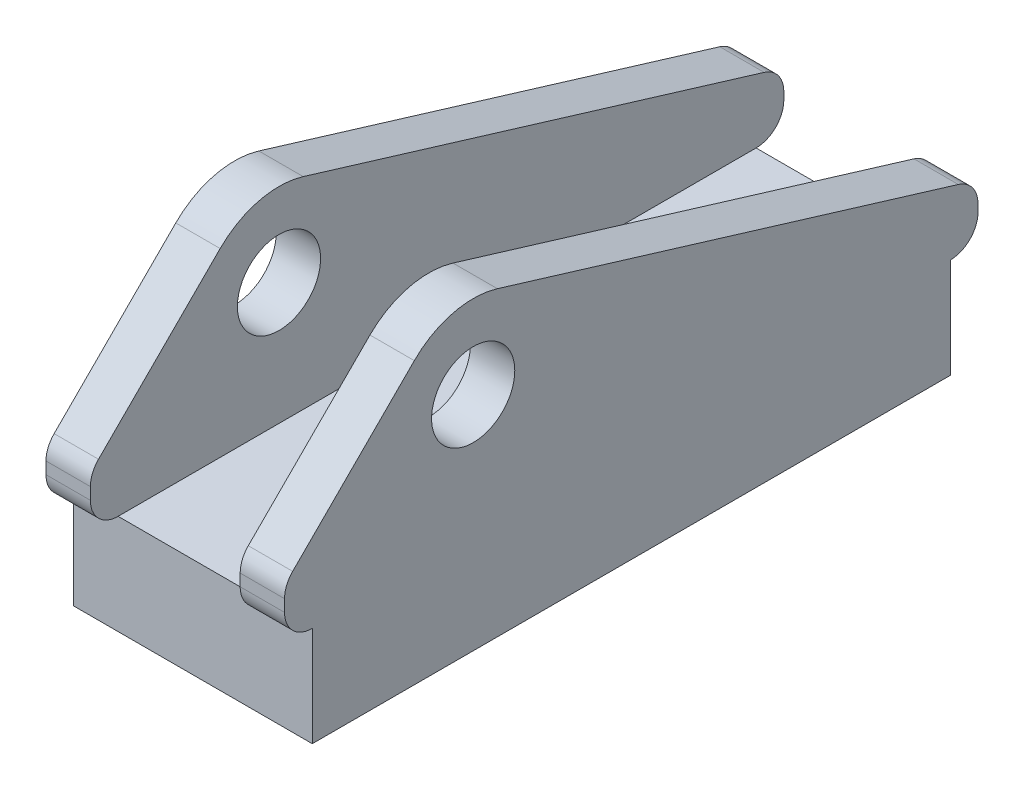
ISO-10303-21;
HEADER;
FILE_DESCRIPTION(('STEP AP214'),'2;1');
FILE_NAME('part.step','',(''),(''),'','','');
FILE_SCHEMA(('AUTOMOTIVE_DESIGN { 1 0 10303 214 1 1 1 1 }'));
ENDSEC;
DATA;
#1=APPLICATION_CONTEXT('core data for automotive mechanical design processes');
#2=APPLICATION_PROTOCOL_DEFINITION('international standard','automotive_design',2000,#1);
#3=PRODUCT_CONTEXT('',#1,'mechanical');
#4=PRODUCT('Part','Part','',(#3));
#5=PRODUCT_RELATED_PRODUCT_CATEGORY('part','',(#4));
#6=PRODUCT_DEFINITION_FORMATION('','',#4);
#7=PRODUCT_DEFINITION_CONTEXT('part definition',#1,'design');
#8=PRODUCT_DEFINITION('design','',#6,#7);
#9=PRODUCT_DEFINITION_SHAPE('','',#8);
#10=(LENGTH_UNIT() NAMED_UNIT(*) SI_UNIT(.MILLI.,.METRE.));
#11=(NAMED_UNIT(*) PLANE_ANGLE_UNIT() SI_UNIT($,.RADIAN.));
#12=(NAMED_UNIT(*) SI_UNIT($,.STERADIAN.) SOLID_ANGLE_UNIT());
#13=UNCERTAINTY_MEASURE_WITH_UNIT(LENGTH_MEASURE(1.E-05),#10,'distance_accuracy_value','');
#14=(GEOMETRIC_REPRESENTATION_CONTEXT(3) GLOBAL_UNCERTAINTY_ASSIGNED_CONTEXT((#13)) GLOBAL_UNIT_ASSIGNED_CONTEXT((#10,
#11,#12)) REPRESENTATION_CONTEXT('',''));
#15=CARTESIAN_POINT('',(0.,0.,0.));
#16=DIRECTION('',(0.,0.,1.));
#17=DIRECTION('',(1.,0.,0.));
#18=AXIS2_PLACEMENT_3D('',#15,#16,#17);
#19=CARTESIAN_POINT('',(43.,18.,-120.));
#20=DIRECTION('',(0.,0.,1.));
#21=DIRECTION('',(0.,-1.,0.));
#22=AXIS2_PLACEMENT_3D('',#19,#20,#21);
#23=PLANE('',#22);
#24=DIRECTION('',(0.,1.,0.));
#25=VECTOR('',#24,1.);
#26=CARTESIAN_POINT('',(0.,18.,-120.));
#27=LINE('',#26,#25);
#28=CARTESIAN_POINT('',(0.,23.,-120.));
#29=VERTEX_POINT('',#28);
#30=CARTESIAN_POINT('',(0.,24.294629651822,-120.));
#31=VERTEX_POINT('',#30);
#32=EDGE_CURVE('E357',#29,#31,#27,.T.);
#33=ORIENTED_EDGE('',*,*,#32,.T.);
#34=DIRECTION('',(-1.,0.,0.));
#35=VECTOR('',#34,1.);
#36=CARTESIAN_POINT('',(43.,24.294629651822,-120.));
#37=LINE('',#36,#35);
#38=CARTESIAN_POINT('',(8.,24.294629651822,-120.));
#39=VERTEX_POINT('',#38);
#40=EDGE_CURVE('E261',#31,#39,#37,.F.);
#41=ORIENTED_EDGE('',*,*,#40,.T.);
#42=DIRECTION('',(0.,-1.,0.));
#43=VECTOR('',#42,1.);
#44=CARTESIAN_POINT('',(8.,18.,-120.));
#45=LINE('',#44,#43);
#46=CARTESIAN_POINT('',(8.,23.,-120.));
#47=VERTEX_POINT('',#46);
#48=EDGE_CURVE('E221',#39,#47,#45,.T.);
#49=ORIENTED_EDGE('',*,*,#48,.T.);
#50=DIRECTION('',(-1.,0.,0.));
#51=VECTOR('',#50,1.);
#52=CARTESIAN_POINT('',(43.,23.,-120.));
#53=LINE('',#52,#51);
#54=EDGE_CURVE('E256',#47,#29,#53,.T.);
#55=ORIENTED_EDGE('',*,*,#54,.T.);
#56=EDGE_LOOP('',(#33,#41,#49,#55));
#57=FACE_BOUND('',#56,.T.);
#58=ADVANCED_FACE('F39',(#57),#23,.F.);
#59=CARTESIAN_POINT('',(43.,28.,-120.));
#60=DIRECTION('',(0.,-0.956724092071816,0.29099658356991));
#61=DIRECTION('',(0.,-0.29099658356991,-0.956724092071816));
#62=AXIS2_PLACEMENT_3D('',#59,#60,#61);
#63=PLANE('',#62);
#64=DIRECTION('',(0.,-0.29099658356991,-0.956724092071816));
#65=VECTOR('',#64,1.);
#66=CARTESIAN_POINT('',(8.,28.,-120.));
#67=LINE('',#66,#65);
#68=CARTESIAN_POINT('',(8.,54.3508613810772,-33.3649487535486));
#69=VERTEX_POINT('',#68);
#70=CARTESIAN_POINT('',(8.,29.078250112181,-116.45498291785));
#71=VERTEX_POINT('',#70);
#72=EDGE_CURVE('E325',#69,#71,#67,.T.);
#73=ORIENTED_EDGE('',*,*,#72,.T.);
#74=DIRECTION('',(-1.,0.,0.));
#75=VECTOR('',#74,1.);
#76=CARTESIAN_POINT('',(43.,29.078250112181,-116.45498291785));
#77=LINE('',#76,#75);
#78=CARTESIAN_POINT('',(0.,29.078250112181,-116.45498291785));
#79=VERTEX_POINT('',#78);
#80=EDGE_CURVE('E239',#71,#79,#77,.T.);
#81=ORIENTED_EDGE('',*,*,#80,.T.);
#82=DIRECTION('',(0.,0.29099658356991,0.956724092071816));
#83=VECTOR('',#82,1.);
#84=CARTESIAN_POINT('',(0.,28.,-120.));
#85=LINE('',#84,#83);
#86=CARTESIAN_POINT('',(0.,54.3508613810772,-33.3649487535486));
#87=VERTEX_POINT('',#86);
#88=EDGE_CURVE('E363',#79,#87,#85,.T.);
#89=ORIENTED_EDGE('',*,*,#88,.T.);
#90=DIRECTION('',(-1.,0.,0.));
#91=VECTOR('',#90,1.);
#92=CARTESIAN_POINT('',(43.,54.3508613810772,-33.3649487535486));
#93=LINE('',#92,#91);
#94=EDGE_CURVE('E374',#69,#87,#93,.T.);
#95=ORIENTED_EDGE('',*,*,#94,.F.);
#96=EDGE_LOOP('',(#73,#81,#89,#95));
#97=FACE_BOUND('',#96,.T.);
#98=ADVANCED_FACE('F459',(#97),#63,.F.);
#99=CARTESIAN_POINT('',(43.,40.,-29.));
#100=DIRECTION('',(-1.,0.,0.));
#101=DIRECTION('',(0.,0.,1.));
#102=AXIS2_PLACEMENT_3D('',#99,#100,#101);
#103=CYLINDRICAL_SURFACE('',#102,15.);
#104=DIRECTION('',(-1.,0.,0.));
#105=VECTOR('',#104,1.);
#106=CARTESIAN_POINT('',(43.,50.6066017177982,-18.3933982822018));
#107=LINE('',#106,#105);
#108=CARTESIAN_POINT('',(8.,50.6066017177982,-18.3933982822018));
#109=VERTEX_POINT('',#108);
#110=CARTESIAN_POINT('',(0.,50.6066017177982,-18.3933982822018));
#111=VERTEX_POINT('',#110);
#112=EDGE_CURVE('E375',#109,#111,#107,.T.);
#113=ORIENTED_EDGE('',*,*,#112,.F.);
#114=CARTESIAN_POINT('',(8.,40.,-29.));
#115=DIRECTION('',(-1.,0.,0.));
#116=DIRECTION('',(0.,0.,1.));
#117=AXIS2_PLACEMENT_3D('',#114,#115,#116);
#118=CIRCLE('',#117,15.);
#119=EDGE_CURVE('E317',#109,#69,#118,.T.);
#120=ORIENTED_EDGE('',*,*,#119,.T.);
#121=ORIENTED_EDGE('',*,*,#94,.T.);
#122=CARTESIAN_POINT('',(0.,40.,-29.));
#123=DIRECTION('',(1.,0.,0.));
#124=DIRECTION('',(0.,0.,-1.));
#125=AXIS2_PLACEMENT_3D('',#122,#123,#124);
#126=CIRCLE('',#125,15.);
#127=EDGE_CURVE('E361',#87,#111,#126,.T.);
#128=ORIENTED_EDGE('',*,*,#127,.T.);
#129=EDGE_LOOP('',(#113,#120,#121,#128));
#130=FACE_BOUND('',#129,.T.);
#131=ADVANCED_FACE('F386',(#130),#103,.T.);
#132=CARTESIAN_POINT('',(43.,50.6066017177982,-18.3933982822018));
#133=DIRECTION('',(0.,-0.707106781186546,-0.707106781186549));
#134=DIRECTION('',(0.,0.707106781186549,-0.707106781186546));
#135=AXIS2_PLACEMENT_3D('',#132,#133,#134);
#136=PLANE('',#135);
#137=DIRECTION('',(0.,-0.707106781186549,0.707106781186546));
#138=VECTOR('',#137,1.);
#139=CARTESIAN_POINT('',(0.,50.6066017177982,-18.3933982822018));
#140=LINE('',#139,#138);
#141=CARTESIAN_POINT('',(0.,28.6776695296636,3.53553390593275));
#142=VERTEX_POINT('',#141);
#143=EDGE_CURVE('E368',#111,#142,#140,.T.);
#144=ORIENTED_EDGE('',*,*,#143,.T.);
#145=DIRECTION('',(-1.,0.,0.));
#146=VECTOR('',#145,1.);
#147=CARTESIAN_POINT('',(43.,28.6776695296636,3.53553390593275));
#148=LINE('',#147,#146);
#149=CARTESIAN_POINT('',(8.,28.6776695296636,3.53553390593275));
#150=VERTEX_POINT('',#149);
#151=EDGE_CURVE('E294',#142,#150,#148,.F.);
#152=ORIENTED_EDGE('',*,*,#151,.T.);
#153=DIRECTION('',(0.,0.707106781186549,-0.707106781186546));
#154=VECTOR('',#153,1.);
#155=CARTESIAN_POINT('',(8.,50.6066017177982,-18.3933982822018));
#156=LINE('',#155,#154);
#157=EDGE_CURVE('E320',#150,#109,#156,.T.);
#158=ORIENTED_EDGE('',*,*,#157,.T.);
#159=ORIENTED_EDGE('',*,*,#112,.T.);
#160=EDGE_LOOP('',(#144,#152,#158,#159));
#161=FACE_BOUND('',#160,.T.);
#162=ADVANCED_FACE('F385',(#161),#136,.F.);
#163=CARTESIAN_POINT('',(43.,27.2132034355963,5.));
#164=DIRECTION('',(0.,0.,-1.));
#165=DIRECTION('',(0.,1.,0.));
#166=AXIS2_PLACEMENT_3D('',#163,#164,#165);
#167=PLANE('',#166);
#168=DIRECTION('',(0.,-1.,0.));
#169=VECTOR('',#168,1.);
#170=CARTESIAN_POINT('',(0.,27.2132034355963,5.));
#171=LINE('',#170,#169);
#172=CARTESIAN_POINT('',(0.,25.1421356237309,5.));
#173=VERTEX_POINT('',#172);
#174=CARTESIAN_POINT('',(0.,23.,5.));
#175=VERTEX_POINT('',#174);
#176=EDGE_CURVE('E340',#173,#175,#171,.T.);
#177=ORIENTED_EDGE('',*,*,#176,.T.);
#178=DIRECTION('',(-1.,0.,0.));
#179=VECTOR('',#178,1.);
#180=CARTESIAN_POINT('',(43.,23.,5.));
#181=LINE('',#180,#179);
#182=CARTESIAN_POINT('',(8.,23.,5.));
#183=VERTEX_POINT('',#182);
#184=EDGE_CURVE('E295',#175,#183,#181,.F.);
#185=ORIENTED_EDGE('',*,*,#184,.T.);
#186=DIRECTION('',(0.,1.,0.));
#187=VECTOR('',#186,1.);
#188=CARTESIAN_POINT('',(8.,27.2132034355963,5.));
#189=LINE('',#188,#187);
#190=CARTESIAN_POINT('',(8.,25.1421356237309,5.));
#191=VERTEX_POINT('',#190);
#192=EDGE_CURVE('E250',#183,#191,#189,.T.);
#193=ORIENTED_EDGE('',*,*,#192,.T.);
#194=DIRECTION('',(-1.,0.,0.));
#195=VECTOR('',#194,1.);
#196=CARTESIAN_POINT('',(43.,25.1421356237309,5.));
#197=LINE('',#196,#195);
#198=EDGE_CURVE('E288',#191,#173,#197,.T.);
#199=ORIENTED_EDGE('',*,*,#198,.T.);
#200=EDGE_LOOP('',(#177,#185,#193,#199));
#201=FACE_BOUND('',#200,.T.);
#202=ADVANCED_FACE('F402',(#201),#167,.F.);
#203=CARTESIAN_POINT('',(43.,40.,-29.));
#204=DIRECTION('',(-1.,0.,0.));
#205=DIRECTION('',(0.,0.,1.));
#206=AXIS2_PLACEMENT_3D('',#203,#204,#205);
#207=CYLINDRICAL_SURFACE('',#206,7.5);
#208=CARTESIAN_POINT('',(8.,40.,-29.));
#209=DIRECTION('',(-1.,0.,0.));
#210=DIRECTION('',(0.,0.,1.));
#211=AXIS2_PLACEMENT_3D('',#208,#209,#210);
#212=CIRCLE('',#211,7.5);
#213=CARTESIAN_POINT('',(8.,40.,-21.5));
#214=VERTEX_POINT('',#213);
#215=EDGE_CURVE('E242',#214,#214,#212,.T.);
#216=ORIENTED_EDGE('',*,*,#215,.F.);
#217=EDGE_LOOP('',(#216));
#218=FACE_BOUND('',#217,.T.);
#219=CARTESIAN_POINT('',(0.,40.,-29.));
#220=DIRECTION('',(1.,0.,0.));
#221=DIRECTION('',(0.,0.,-1.));
#222=AXIS2_PLACEMENT_3D('',#219,#220,#221);
#223=CIRCLE('',#222,7.5);
#224=CARTESIAN_POINT('',(0.,40.,-36.5));
#225=VERTEX_POINT('',#224);
#226=EDGE_CURVE('E224',#225,#225,#223,.T.);
#227=ORIENTED_EDGE('',*,*,#226,.F.);
#228=EDGE_LOOP('',(#227));
#229=FACE_BOUND('',#228,.T.);
#230=ADVANCED_FACE('F600',(#218,#229),#207,.F.);
#231=CARTESIAN_POINT('',(43.,40.,-29.));
#232=DIRECTION('',(1.,0.,0.));
#233=DIRECTION('',(0.,0.,-1.));
#234=AXIS2_PLACEMENT_3D('',#231,#232,#233);
#235=PLANE('',#234);
#236=DIRECTION('',(0.,1.,0.));
#237=VECTOR('',#236,1.);
#238=CARTESIAN_POINT('',(43.,0.,-115.));
#239=LINE('',#238,#237);
#240=CARTESIAN_POINT('',(43.,0.,-115.));
#241=VERTEX_POINT('',#240);
#242=CARTESIAN_POINT('',(43.,18.,-115.));
#243=VERTEX_POINT('',#242);
#244=EDGE_CURVE('E337',#241,#243,#239,.T.);
#245=ORIENTED_EDGE('',*,*,#244,.T.);
#246=CARTESIAN_POINT('',(43.,23.,-115.));
#247=DIRECTION('',(1.,0.,0.));
#248=DIRECTION('',(0.,0.,-1.));
#249=AXIS2_PLACEMENT_3D('',#246,#247,#248);
#250=CIRCLE('',#249,5.);
#251=CARTESIAN_POINT('',(43.,23.,-120.));
#252=VERTEX_POINT('',#251);
#253=EDGE_CURVE('E230',#243,#252,#250,.T.);
#254=ORIENTED_EDGE('',*,*,#253,.T.);
#255=DIRECTION('',(0.,1.,0.));
#256=VECTOR('',#255,1.);
#257=CARTESIAN_POINT('',(43.,18.,-120.));
#258=LINE('',#257,#256);
#259=CARTESIAN_POINT('',(43.,24.294629651822,-120.));
#260=VERTEX_POINT('',#259);
#261=EDGE_CURVE('E341',#252,#260,#258,.T.);
#262=ORIENTED_EDGE('',*,*,#261,.T.);
#263=CARTESIAN_POINT('',(43.,24.294629651822,-115.));
#264=DIRECTION('',(1.,0.,0.));
#265=DIRECTION('',(0.,0.,-1.));
#266=AXIS2_PLACEMENT_3D('',#263,#264,#265);
#267=CIRCLE('',#266,5.);
#268=CARTESIAN_POINT('',(43.,29.078250112181,-116.45498291785));
#269=VERTEX_POINT('',#268);
#270=EDGE_CURVE('E281',#260,#269,#267,.T.);
#271=ORIENTED_EDGE('',*,*,#270,.T.);
#272=DIRECTION('',(0.,0.29099658356991,0.956724092071816));
#273=VECTOR('',#272,1.);
#274=CARTESIAN_POINT('',(43.,28.,-120.));
#275=LINE('',#274,#273);
#276=CARTESIAN_POINT('',(43.,54.3508613810772,-33.3649487535486));
#277=VERTEX_POINT('',#276);
#278=EDGE_CURVE('E343',#269,#277,#275,.T.);
#279=ORIENTED_EDGE('',*,*,#278,.T.);
#280=CARTESIAN_POINT('',(43.,40.,-29.));
#281=DIRECTION('',(1.,0.,0.));
#282=DIRECTION('',(0.,0.,-1.));
#283=AXIS2_PLACEMENT_3D('',#280,#281,#282);
#284=CIRCLE('',#283,15.);
#285=CARTESIAN_POINT('',(43.,50.6066017177982,-18.3933982822018));
#286=VERTEX_POINT('',#285);
#287=EDGE_CURVE('E347',#277,#286,#284,.T.);
#288=ORIENTED_EDGE('',*,*,#287,.T.);
#289=DIRECTION('',(0.,-0.707106781186549,0.707106781186546));
#290=VECTOR('',#289,1.);
#291=CARTESIAN_POINT('',(43.,50.6066017177982,-18.3933982822018));
#292=LINE('',#291,#290);
#293=CARTESIAN_POINT('',(43.,28.6776695296636,3.53553390593275));
#294=VERTEX_POINT('',#293);
#295=EDGE_CURVE('E346',#286,#294,#292,.T.);
#296=ORIENTED_EDGE('',*,*,#295,.T.);
#297=CARTESIAN_POINT('',(43.,25.1421356237309,0.));
#298=DIRECTION('',(1.,0.,0.));
#299=DIRECTION('',(0.,0.,-1.));
#300=AXIS2_PLACEMENT_3D('',#297,#298,#299);
#301=CIRCLE('',#300,5.);
#302=CARTESIAN_POINT('',(43.,25.1421356237309,5.));
#303=VERTEX_POINT('',#302);
#304=EDGE_CURVE('E58',#294,#303,#301,.T.);
#305=ORIENTED_EDGE('',*,*,#304,.T.);
#306=DIRECTION('',(0.,-1.,0.));
#307=VECTOR('',#306,1.);
#308=CARTESIAN_POINT('',(43.,27.2132034355963,5.));
#309=LINE('',#308,#307);
#310=CARTESIAN_POINT('',(43.,23.,5.));
#311=VERTEX_POINT('',#310);
#312=EDGE_CURVE('E301',#303,#311,#309,.T.);
#313=ORIENTED_EDGE('',*,*,#312,.T.);
#314=CARTESIAN_POINT('',(43.,23.,0.));
#315=DIRECTION('',(1.,0.,0.));
#316=DIRECTION('',(0.,0.,-1.));
#317=AXIS2_PLACEMENT_3D('',#314,#315,#316);
#318=CIRCLE('',#317,5.);
#319=CARTESIAN_POINT('',(43.,18.,0.));
#320=VERTEX_POINT('',#319);
#321=EDGE_CURVE('E283',#311,#320,#318,.T.);
#322=ORIENTED_EDGE('',*,*,#321,.T.);
#323=DIRECTION('',(0.,-1.,0.));
#324=VECTOR('',#323,1.);
#325=CARTESIAN_POINT('',(43.,18.,0.));
#326=LINE('',#325,#324);
#327=CARTESIAN_POINT('',(43.,0.,0.));
#328=VERTEX_POINT('',#327);
#329=EDGE_CURVE('E334',#320,#328,#326,.T.);
#330=ORIENTED_EDGE('',*,*,#329,.T.);
#331=DIRECTION('',(0.,0.,-1.));
#332=VECTOR('',#331,1.);
#333=CARTESIAN_POINT('',(43.,0.,0.));
#334=LINE('',#333,#332);
#335=EDGE_CURVE('E338',#328,#241,#334,.T.);
#336=ORIENTED_EDGE('',*,*,#335,.T.);
#337=EDGE_LOOP('',(#245,#254,#262,#271,#279,#288,#296,#305,#313,#322,#330,#336));
#338=FACE_BOUND('',#337,.T.);
#339=CARTESIAN_POINT('',(43.,40.,-29.));
#340=DIRECTION('',(1.,0.,0.));
#341=DIRECTION('',(0.,0.,-1.));
#342=AXIS2_PLACEMENT_3D('',#339,#340,#341);
#343=CIRCLE('',#342,7.5);
#344=CARTESIAN_POINT('',(43.,40.,-36.5));
#345=VERTEX_POINT('',#344);
#346=EDGE_CURVE('E330',#345,#345,#343,.T.);
#347=ORIENTED_EDGE('',*,*,#346,.F.);
#348=EDGE_LOOP('',(#347));
#349=FACE_BOUND('',#348,.T.);
#350=ADVANCED_FACE('F423',(#338,#349),#235,.T.);
#351=CARTESIAN_POINT('',(0.,40.,-29.));
#352=DIRECTION('',(1.,0.,0.));
#353=DIRECTION('',(0.,0.,-1.));
#354=AXIS2_PLACEMENT_3D('',#351,#352,#353);
#355=PLANE('',#354);
#356=ORIENTED_EDGE('',*,*,#88,.F.);
#357=CARTESIAN_POINT('',(0.,24.294629651822,-115.));
#358=DIRECTION('',(1.,0.,0.));
#359=DIRECTION('',(0.,0.,-1.));
#360=AXIS2_PLACEMENT_3D('',#357,#358,#359);
#361=CIRCLE('',#360,5.);
#362=EDGE_CURVE('E258',#79,#31,#361,.F.);
#363=ORIENTED_EDGE('',*,*,#362,.T.);
#364=ORIENTED_EDGE('',*,*,#32,.F.);
#365=CARTESIAN_POINT('',(0.,23.,-115.));
#366=DIRECTION('',(1.,0.,0.));
#367=DIRECTION('',(0.,0.,-1.));
#368=AXIS2_PLACEMENT_3D('',#365,#366,#367);
#369=CIRCLE('',#368,5.);
#370=CARTESIAN_POINT('',(0.,18.,-115.));
#371=VERTEX_POINT('',#370);
#372=EDGE_CURVE('E255',#29,#371,#369,.F.);
#373=ORIENTED_EDGE('',*,*,#372,.T.);
#374=DIRECTION('',(0.,1.,0.));
#375=VECTOR('',#374,1.);
#376=CARTESIAN_POINT('',(0.,0.,-115.));
#377=LINE('',#376,#375);
#378=CARTESIAN_POINT('',(0.,0.,-115.));
#379=VERTEX_POINT('',#378);
#380=EDGE_CURVE('E356',#379,#371,#377,.T.);
#381=ORIENTED_EDGE('',*,*,#380,.F.);
#382=DIRECTION('',(0.,0.,-1.));
#383=VECTOR('',#382,1.);
#384=CARTESIAN_POINT('',(0.,0.,0.));
#385=LINE('',#384,#383);
#386=CARTESIAN_POINT('',(0.,0.,0.));
#387=VERTEX_POINT('',#386);
#388=EDGE_CURVE('E352',#387,#379,#385,.T.);
#389=ORIENTED_EDGE('',*,*,#388,.F.);
#390=DIRECTION('',(0.,-1.,0.));
#391=VECTOR('',#390,1.);
#392=CARTESIAN_POINT('',(0.,18.,0.));
#393=LINE('',#392,#391);
#394=CARTESIAN_POINT('',(0.,18.,0.));
#395=VERTEX_POINT('',#394);
#396=EDGE_CURVE('E329',#395,#387,#393,.T.);
#397=ORIENTED_EDGE('',*,*,#396,.F.);
#398=CARTESIAN_POINT('',(0.,23.,0.));
#399=DIRECTION('',(1.,0.,0.));
#400=DIRECTION('',(0.,0.,-1.));
#401=AXIS2_PLACEMENT_3D('',#398,#399,#400);
#402=CIRCLE('',#401,5.);
#403=EDGE_CURVE('E252',#395,#175,#402,.F.);
#404=ORIENTED_EDGE('',*,*,#403,.T.);
#405=ORIENTED_EDGE('',*,*,#176,.F.);
#406=CARTESIAN_POINT('',(0.,25.1421356237309,0.));
#407=DIRECTION('',(1.,0.,0.));
#408=DIRECTION('',(0.,0.,-1.));
#409=AXIS2_PLACEMENT_3D('',#406,#407,#408);
#410=CIRCLE('',#409,5.);
#411=EDGE_CURVE('E249',#173,#142,#410,.F.);
#412=ORIENTED_EDGE('',*,*,#411,.T.);
#413=ORIENTED_EDGE('',*,*,#143,.F.);
#414=ORIENTED_EDGE('',*,*,#127,.F.);
#415=EDGE_LOOP('',(#356,#363,#364,#373,#381,#389,#397,#404,#405,#412,#413,#414));
#416=FACE_BOUND('',#415,.T.);
#417=ORIENTED_EDGE('',*,*,#226,.T.);
#418=EDGE_LOOP('',(#417));
#419=FACE_BOUND('',#418,.T.);
#420=ADVANCED_FACE('F391',(#416,#419),#355,.F.);
#421=CARTESIAN_POINT('',(43.,18.,0.));
#422=DIRECTION('',(0.,0.,-1.));
#423=DIRECTION('',(0.,1.,0.));
#424=AXIS2_PLACEMENT_3D('',#421,#422,#423);
#425=PLANE('',#424);
#426=ORIENTED_EDGE('',*,*,#396,.T.);
#427=DIRECTION('',(-1.,0.,0.));
#428=VECTOR('',#427,1.);
#429=CARTESIAN_POINT('',(43.,0.,0.));
#430=LINE('',#429,#428);
#431=EDGE_CURVE('E231',#328,#387,#430,.T.);
#432=ORIENTED_EDGE('',*,*,#431,.F.);
#433=ORIENTED_EDGE('',*,*,#329,.F.);
#434=DIRECTION('',(-1.,0.,0.));
#435=VECTOR('',#434,1.);
#436=CARTESIAN_POINT('',(43.,18.,0.));
#437=LINE('',#436,#435);
#438=CARTESIAN_POINT('',(35.,18.,0.));
#439=VERTEX_POINT('',#438);
#440=EDGE_CURVE('E371',#320,#439,#437,.T.);
#441=ORIENTED_EDGE('',*,*,#440,.T.);
#442=CARTESIAN_POINT('',(8.,18.,0.));
#443=VERTEX_POINT('',#442);
#444=EDGE_CURVE('E208',#439,#443,#437,.T.);
#445=ORIENTED_EDGE('',*,*,#444,.T.);
#446=EDGE_CURVE('E353',#443,#395,#437,.T.);
#447=ORIENTED_EDGE('',*,*,#446,.T.);
#448=EDGE_LOOP('',(#426,#432,#433,#441,#445,#447));
#449=FACE_BOUND('',#448,.T.);
#450=ADVANCED_FACE('F413',(#449),#425,.F.);
#451=CARTESIAN_POINT('',(43.,0.,0.));
#452=DIRECTION('',(0.,1.,0.));
#453=DIRECTION('',(0.,0.,1.));
#454=AXIS2_PLACEMENT_3D('',#451,#452,#453);
#455=PLANE('',#454);
#456=ORIENTED_EDGE('',*,*,#388,.T.);
#457=DIRECTION('',(-1.,0.,0.));
#458=VECTOR('',#457,1.);
#459=CARTESIAN_POINT('',(43.,0.,-115.));
#460=LINE('',#459,#458);
#461=EDGE_CURVE('E226',#241,#379,#460,.T.);
#462=ORIENTED_EDGE('',*,*,#461,.F.);
#463=ORIENTED_EDGE('',*,*,#335,.F.);
#464=ORIENTED_EDGE('',*,*,#431,.T.);
#465=EDGE_LOOP('',(#456,#462,#463,#464));
#466=FACE_BOUND('',#465,.T.);
#467=ADVANCED_FACE('F422',(#466),#455,.F.);
#468=CARTESIAN_POINT('',(43.,0.,-115.));
#469=DIRECTION('',(0.,0.,1.));
#470=DIRECTION('',(1.,0.,0.));
#471=AXIS2_PLACEMENT_3D('',#468,#469,#470);
#472=PLANE('',#471);
#473=ORIENTED_EDGE('',*,*,#380,.T.);
#474=DIRECTION('',(-1.,0.,0.));
#475=VECTOR('',#474,1.);
#476=CARTESIAN_POINT('',(43.,18.,-115.));
#477=LINE('',#476,#475);
#478=CARTESIAN_POINT('',(8.,18.,-115.));
#479=VERTEX_POINT('',#478);
#480=EDGE_CURVE('E222',#479,#371,#477,.T.);
#481=ORIENTED_EDGE('',*,*,#480,.F.);
#482=DIRECTION('',(1.,0.,0.));
#483=VECTOR('',#482,1.);
#484=CARTESIAN_POINT('',(43.,18.,-115.));
#485=LINE('',#484,#483);
#486=CARTESIAN_POINT('',(35.,18.,-115.));
#487=VERTEX_POINT('',#486);
#488=EDGE_CURVE('E202',#479,#487,#485,.T.);
#489=ORIENTED_EDGE('',*,*,#488,.T.);
#490=EDGE_CURVE('E217',#243,#487,#477,.T.);
#491=ORIENTED_EDGE('',*,*,#490,.F.);
#492=ORIENTED_EDGE('',*,*,#244,.F.);
#493=ORIENTED_EDGE('',*,*,#461,.T.);
#494=EDGE_LOOP('',(#473,#481,#489,#491,#492,#493));
#495=FACE_BOUND('',#494,.T.);
#496=ADVANCED_FACE('F216',(#495),#472,.F.);
#497=ORIENTED_EDGE('',*,*,#261,.F.);
#498=DIRECTION('',(-1.,0.,0.));
#499=VECTOR('',#498,1.);
#500=CARTESIAN_POINT('',(43.,23.,-120.));
#501=LINE('',#500,#499);
#502=CARTESIAN_POINT('',(35.,23.,-120.));
#503=VERTEX_POINT('',#502);
#504=EDGE_CURVE('E272',#252,#503,#501,.T.);
#505=ORIENTED_EDGE('',*,*,#504,.T.);
#506=DIRECTION('',(0.,1.,0.));
#507=VECTOR('',#506,1.);
#508=CARTESIAN_POINT('',(35.,18.,-120.));
#509=LINE('',#508,#507);
#510=CARTESIAN_POINT('',(35.,24.294629651822,-120.));
#511=VERTEX_POINT('',#510);
#512=EDGE_CURVE('E193',#503,#511,#509,.T.);
#513=ORIENTED_EDGE('',*,*,#512,.T.);
#514=DIRECTION('',(-1.,0.,0.));
#515=VECTOR('',#514,1.);
#516=CARTESIAN_POINT('',(43.,24.294629651822,-120.));
#517=LINE('',#516,#515);
#518=EDGE_CURVE('E271',#511,#260,#517,.F.);
#519=ORIENTED_EDGE('',*,*,#518,.T.);
#520=EDGE_LOOP('',(#497,#505,#513,#519));
#521=FACE_BOUND('',#520,.T.);
#522=ADVANCED_FACE('F429',(#521),#23,.F.);
#523=ORIENTED_EDGE('',*,*,#278,.F.);
#524=DIRECTION('',(-1.,0.,0.));
#525=VECTOR('',#524,1.);
#526=CARTESIAN_POINT('',(43.,29.078250112181,-116.45498291785));
#527=LINE('',#526,#525);
#528=CARTESIAN_POINT('',(35.,29.078250112181,-116.45498291785));
#529=VERTEX_POINT('',#528);
#530=EDGE_CURVE('E286',#269,#529,#527,.T.);
#531=ORIENTED_EDGE('',*,*,#530,.T.);
#532=DIRECTION('',(0.,0.29099658356991,0.956724092071816));
#533=VECTOR('',#532,1.);
#534=CARTESIAN_POINT('',(35.,28.,-120.));
#535=LINE('',#534,#533);
#536=CARTESIAN_POINT('',(35.,54.3508613810772,-33.3649487535486));
#537=VERTEX_POINT('',#536);
#538=EDGE_CURVE('E315',#529,#537,#535,.T.);
#539=ORIENTED_EDGE('',*,*,#538,.T.);
#540=EDGE_CURVE('E232',#277,#537,#93,.T.);
#541=ORIENTED_EDGE('',*,*,#540,.F.);
#542=EDGE_LOOP('',(#523,#531,#539,#541));
#543=FACE_BOUND('',#542,.T.);
#544=ADVANCED_FACE('F437',(#543),#63,.F.);
#545=ORIENTED_EDGE('',*,*,#540,.T.);
#546=CARTESIAN_POINT('',(35.,40.,-29.));
#547=DIRECTION('',(1.,0.,0.));
#548=DIRECTION('',(0.,0.,-1.));
#549=AXIS2_PLACEMENT_3D('',#546,#547,#548);
#550=CIRCLE('',#549,15.);
#551=CARTESIAN_POINT('',(35.,50.6066017177982,-18.3933982822018));
#552=VERTEX_POINT('',#551);
#553=EDGE_CURVE('E308',#537,#552,#550,.T.);
#554=ORIENTED_EDGE('',*,*,#553,.T.);
#555=EDGE_CURVE('E373',#286,#552,#107,.T.);
#556=ORIENTED_EDGE('',*,*,#555,.F.);
#557=ORIENTED_EDGE('',*,*,#287,.F.);
#558=EDGE_LOOP('',(#545,#554,#556,#557));
#559=FACE_BOUND('',#558,.T.);
#560=ADVANCED_FACE('F441',(#559),#103,.T.);
#561=DIRECTION('',(0.,-0.707106781186549,0.707106781186546));
#562=VECTOR('',#561,1.);
#563=CARTESIAN_POINT('',(35.,50.6066017177982,-18.3933982822018));
#564=LINE('',#563,#562);
#565=CARTESIAN_POINT('',(35.,28.6776695296636,3.53553390593275));
#566=VERTEX_POINT('',#565);
#567=EDGE_CURVE('E303',#552,#566,#564,.T.);
#568=ORIENTED_EDGE('',*,*,#567,.T.);
#569=DIRECTION('',(-1.,0.,0.));
#570=VECTOR('',#569,1.);
#571=CARTESIAN_POINT('',(43.,28.6776695296636,3.53553390593275));
#572=LINE('',#571,#570);
#573=EDGE_CURVE('E11',#566,#294,#572,.F.);
#574=ORIENTED_EDGE('',*,*,#573,.T.);
#575=ORIENTED_EDGE('',*,*,#295,.F.);
#576=ORIENTED_EDGE('',*,*,#555,.T.);
#577=EDGE_LOOP('',(#568,#574,#575,#576));
#578=FACE_BOUND('',#577,.T.);
#579=ADVANCED_FACE('F448',(#578),#136,.F.);
#580=DIRECTION('',(0.,-1.,0.));
#581=VECTOR('',#580,1.);
#582=CARTESIAN_POINT('',(35.,27.2132034355963,5.));
#583=LINE('',#582,#581);
#584=CARTESIAN_POINT('',(35.,25.1421356237309,5.));
#585=VERTEX_POINT('',#584);
#586=CARTESIAN_POINT('',(35.,23.,5.));
#587=VERTEX_POINT('',#586);
#588=EDGE_CURVE('E241',#585,#587,#583,.T.);
#589=ORIENTED_EDGE('',*,*,#588,.T.);
#590=DIRECTION('',(-1.,0.,0.));
#591=VECTOR('',#590,1.);
#592=CARTESIAN_POINT('',(43.,23.,5.));
#593=LINE('',#592,#591);
#594=EDGE_CURVE('E50',#587,#311,#593,.F.);
#595=ORIENTED_EDGE('',*,*,#594,.T.);
#596=ORIENTED_EDGE('',*,*,#312,.F.);
#597=DIRECTION('',(-1.,0.,0.));
#598=VECTOR('',#597,1.);
#599=CARTESIAN_POINT('',(43.,25.1421356237309,5.));
#600=LINE('',#599,#598);
#601=EDGE_CURVE('E298',#303,#585,#600,.T.);
#602=ORIENTED_EDGE('',*,*,#601,.T.);
#603=EDGE_LOOP('',(#589,#595,#596,#602));
#604=FACE_BOUND('',#603,.T.);
#605=ADVANCED_FACE('F299',(#604),#167,.F.);
#606=CARTESIAN_POINT('',(35.,40.,-29.));
#607=DIRECTION('',(1.,0.,0.));
#608=DIRECTION('',(0.,0.,-1.));
#609=AXIS2_PLACEMENT_3D('',#606,#607,#608);
#610=CIRCLE('',#609,7.5);
#611=CARTESIAN_POINT('',(35.,40.,-36.5));
#612=VERTEX_POINT('',#611);
#613=EDGE_CURVE('E238',#612,#612,#610,.T.);
#614=ORIENTED_EDGE('',*,*,#613,.F.);
#615=EDGE_LOOP('',(#614));
#616=FACE_BOUND('',#615,.T.);
#617=ORIENTED_EDGE('',*,*,#346,.T.);
#618=EDGE_LOOP('',(#617));
#619=FACE_BOUND('',#618,.T.);
#620=ADVANCED_FACE('F452',(#616,#619),#207,.F.);
#621=CARTESIAN_POINT('',(35.,18.,74.0000000000001));
#622=DIRECTION('',(0.,-1.,0.));
#623=DIRECTION('',(0.,0.,-1.));
#624=AXIS2_PLACEMENT_3D('',#621,#622,#623);
#625=PLANE('',#624);
#626=DIRECTION('',(0.,0.,-1.));
#627=VECTOR('',#626,1.);
#628=CARTESIAN_POINT('',(35.,18.,74.0000000000001));
#629=LINE('',#628,#627);
#630=EDGE_CURVE('E191',#439,#487,#629,.T.);
#631=ORIENTED_EDGE('',*,*,#630,.T.);
#632=ORIENTED_EDGE('',*,*,#488,.F.);
#633=DIRECTION('',(0.,0.,-1.));
#634=VECTOR('',#633,1.);
#635=CARTESIAN_POINT('',(8.,18.,74.0000000000001));
#636=LINE('',#635,#634);
#637=EDGE_CURVE('E209',#443,#479,#636,.T.);
#638=ORIENTED_EDGE('',*,*,#637,.F.);
#639=ORIENTED_EDGE('',*,*,#444,.F.);
#640=EDGE_LOOP('',(#631,#632,#638,#639));
#641=FACE_BOUND('',#640,.T.);
#642=ADVANCED_FACE('F201',(#641),#625,.F.);
#643=CARTESIAN_POINT('',(8.,18.,74.0000000000001));
#644=DIRECTION('',(-1.,0.,0.));
#645=DIRECTION('',(0.,0.,1.));
#646=AXIS2_PLACEMENT_3D('',#643,#644,#645);
#647=PLANE('',#646);
#648=ORIENTED_EDGE('',*,*,#215,.T.);
#649=EDGE_LOOP('',(#648));
#650=FACE_BOUND('',#649,.T.);
#651=ORIENTED_EDGE('',*,*,#48,.F.);
#652=CARTESIAN_POINT('',(8.,24.294629651822,-115.));
#653=DIRECTION('',(-1.,0.,0.));
#654=DIRECTION('',(0.,0.,1.));
#655=AXIS2_PLACEMENT_3D('',#652,#653,#654);
#656=CIRCLE('',#655,5.);
#657=EDGE_CURVE('E267',#39,#71,#656,.F.);
#658=ORIENTED_EDGE('',*,*,#657,.T.);
#659=ORIENTED_EDGE('',*,*,#72,.F.);
#660=ORIENTED_EDGE('',*,*,#119,.F.);
#661=ORIENTED_EDGE('',*,*,#157,.F.);
#662=CARTESIAN_POINT('',(8.,25.1421356237309,0.));
#663=DIRECTION('',(-1.,0.,0.));
#664=DIRECTION('',(0.,0.,1.));
#665=AXIS2_PLACEMENT_3D('',#662,#663,#664);
#666=CIRCLE('',#665,5.);
#667=EDGE_CURVE('E263',#150,#191,#666,.F.);
#668=ORIENTED_EDGE('',*,*,#667,.T.);
#669=ORIENTED_EDGE('',*,*,#192,.F.);
#670=CARTESIAN_POINT('',(8.,23.,0.));
#671=DIRECTION('',(-1.,0.,0.));
#672=DIRECTION('',(0.,0.,1.));
#673=AXIS2_PLACEMENT_3D('',#670,#671,#672);
#674=CIRCLE('',#673,5.);
#675=EDGE_CURVE('E264',#183,#443,#674,.F.);
#676=ORIENTED_EDGE('',*,*,#675,.T.);
#677=ORIENTED_EDGE('',*,*,#637,.T.);
#678=CARTESIAN_POINT('',(8.,23.,-115.));
#679=DIRECTION('',(-1.,0.,0.));
#680=DIRECTION('',(0.,0.,1.));
#681=AXIS2_PLACEMENT_3D('',#678,#679,#680);
#682=CIRCLE('',#681,5.);
#683=EDGE_CURVE('E270',#479,#47,#682,.F.);
#684=ORIENTED_EDGE('',*,*,#683,.T.);
#685=EDGE_LOOP('',(#651,#658,#659,#660,#661,#668,#669,#676,#677,#684));
#686=FACE_BOUND('',#685,.T.);
#687=ADVANCED_FACE('F410',(#650,#686),#647,.F.);
#688=CARTESIAN_POINT('',(35.,18.,74.0000000000001));
#689=DIRECTION('',(1.,0.,0.));
#690=DIRECTION('',(0.,0.,-1.));
#691=AXIS2_PLACEMENT_3D('',#688,#689,#690);
#692=PLANE('',#691);
#693=ORIENTED_EDGE('',*,*,#613,.T.);
#694=EDGE_LOOP('',(#693));
#695=FACE_BOUND('',#694,.T.);
#696=ORIENTED_EDGE('',*,*,#512,.F.);
#697=CARTESIAN_POINT('',(35.,23.,-115.));
#698=DIRECTION('',(1.,0.,0.));
#699=DIRECTION('',(0.,0.,-1.));
#700=AXIS2_PLACEMENT_3D('',#697,#698,#699);
#701=CIRCLE('',#700,5.);
#702=EDGE_CURVE('E186',#503,#487,#701,.F.);
#703=ORIENTED_EDGE('',*,*,#702,.T.);
#704=ORIENTED_EDGE('',*,*,#630,.F.);
#705=CARTESIAN_POINT('',(35.,23.,0.));
#706=DIRECTION('',(1.,0.,0.));
#707=DIRECTION('',(0.,0.,-1.));
#708=AXIS2_PLACEMENT_3D('',#705,#706,#707);
#709=CIRCLE('',#708,5.);
#710=EDGE_CURVE('E280',#439,#587,#709,.F.);
#711=ORIENTED_EDGE('',*,*,#710,.T.);
#712=ORIENTED_EDGE('',*,*,#588,.F.);
#713=CARTESIAN_POINT('',(35.,25.1421356237309,0.));
#714=DIRECTION('',(1.,0.,0.));
#715=DIRECTION('',(0.,0.,-1.));
#716=AXIS2_PLACEMENT_3D('',#713,#714,#715);
#717=CIRCLE('',#716,5.);
#718=EDGE_CURVE('E274',#585,#566,#717,.F.);
#719=ORIENTED_EDGE('',*,*,#718,.T.);
#720=ORIENTED_EDGE('',*,*,#567,.F.);
#721=ORIENTED_EDGE('',*,*,#553,.F.);
#722=ORIENTED_EDGE('',*,*,#538,.F.);
#723=CARTESIAN_POINT('',(35.,24.294629651822,-115.));
#724=DIRECTION('',(1.,0.,0.));
#725=DIRECTION('',(0.,0.,-1.));
#726=AXIS2_PLACEMENT_3D('',#723,#724,#725);
#727=CIRCLE('',#726,5.);
#728=EDGE_CURVE('E200',#529,#511,#727,.F.);
#729=ORIENTED_EDGE('',*,*,#728,.T.);
#730=EDGE_LOOP('',(#696,#703,#704,#711,#712,#719,#720,#721,#722,#729));
#731=FACE_BOUND('',#730,.T.);
#732=ADVANCED_FACE('F189',(#695,#731),#692,.F.);
#733=CARTESIAN_POINT('',(43.,24.294629651822,-115.));
#734=DIRECTION('',(-1.,0.,0.));
#735=DIRECTION('',(0.,0.,1.));
#736=AXIS2_PLACEMENT_3D('',#733,#734,#735);
#737=CYLINDRICAL_SURFACE('',#736,5.);
#738=ORIENTED_EDGE('',*,*,#657,.F.);
#739=ORIENTED_EDGE('',*,*,#40,.F.);
#740=ORIENTED_EDGE('',*,*,#362,.F.);
#741=ORIENTED_EDGE('',*,*,#80,.F.);
#742=EDGE_LOOP('',(#738,#739,#740,#741));
#743=FACE_BOUND('',#742,.T.);
#744=ADVANCED_FACE('F477',(#743),#737,.T.);
#745=CARTESIAN_POINT('',(43.,23.,-115.));
#746=DIRECTION('',(-1.,0.,0.));
#747=DIRECTION('',(0.,0.,1.));
#748=AXIS2_PLACEMENT_3D('',#745,#746,#747);
#749=CYLINDRICAL_SURFACE('',#748,5.);
#750=ORIENTED_EDGE('',*,*,#683,.F.);
#751=ORIENTED_EDGE('',*,*,#480,.T.);
#752=ORIENTED_EDGE('',*,*,#372,.F.);
#753=ORIENTED_EDGE('',*,*,#54,.F.);
#754=EDGE_LOOP('',(#750,#751,#752,#753));
#755=FACE_BOUND('',#754,.T.);
#756=ADVANCED_FACE('F483',(#755),#749,.T.);
#757=CARTESIAN_POINT('',(43.,23.,-115.));
#758=DIRECTION('',(-1.,0.,0.));
#759=DIRECTION('',(0.,0.,1.));
#760=AXIS2_PLACEMENT_3D('',#757,#758,#759);
#761=CYLINDRICAL_SURFACE('',#760,5.);
#762=ORIENTED_EDGE('',*,*,#253,.F.);
#763=ORIENTED_EDGE('',*,*,#490,.T.);
#764=ORIENTED_EDGE('',*,*,#702,.F.);
#765=ORIENTED_EDGE('',*,*,#504,.F.);
#766=EDGE_LOOP('',(#762,#763,#764,#765));
#767=FACE_BOUND('',#766,.T.);
#768=ADVANCED_FACE('F228',(#767),#761,.T.);
#769=CARTESIAN_POINT('',(43.,24.294629651822,-115.));
#770=DIRECTION('',(-1.,0.,0.));
#771=DIRECTION('',(0.,0.,1.));
#772=AXIS2_PLACEMENT_3D('',#769,#770,#771);
#773=CYLINDRICAL_SURFACE('',#772,5.);
#774=ORIENTED_EDGE('',*,*,#270,.F.);
#775=ORIENTED_EDGE('',*,*,#518,.F.);
#776=ORIENTED_EDGE('',*,*,#728,.F.);
#777=ORIENTED_EDGE('',*,*,#530,.F.);
#778=EDGE_LOOP('',(#774,#775,#776,#777));
#779=FACE_BOUND('',#778,.T.);
#780=ADVANCED_FACE('F433',(#779),#773,.T.);
#781=CARTESIAN_POINT('',(43.,23.,0.));
#782=DIRECTION('',(-1.,0.,0.));
#783=DIRECTION('',(0.,0.,1.));
#784=AXIS2_PLACEMENT_3D('',#781,#782,#783);
#785=CYLINDRICAL_SURFACE('',#784,5.);
#786=ORIENTED_EDGE('',*,*,#675,.F.);
#787=ORIENTED_EDGE('',*,*,#184,.F.);
#788=ORIENTED_EDGE('',*,*,#403,.F.);
#789=ORIENTED_EDGE('',*,*,#446,.F.);
#790=EDGE_LOOP('',(#786,#787,#788,#789));
#791=FACE_BOUND('',#790,.T.);
#792=ADVANCED_FACE('F409',(#791),#785,.T.);
#793=CARTESIAN_POINT('',(43.,25.1421356237309,0.));
#794=DIRECTION('',(-1.,0.,0.));
#795=DIRECTION('',(0.,0.,1.));
#796=AXIS2_PLACEMENT_3D('',#793,#794,#795);
#797=CYLINDRICAL_SURFACE('',#796,5.);
#798=ORIENTED_EDGE('',*,*,#667,.F.);
#799=ORIENTED_EDGE('',*,*,#151,.F.);
#800=ORIENTED_EDGE('',*,*,#411,.F.);
#801=ORIENTED_EDGE('',*,*,#198,.F.);
#802=EDGE_LOOP('',(#798,#799,#800,#801));
#803=FACE_BOUND('',#802,.T.);
#804=ADVANCED_FACE('F398',(#803),#797,.T.);
#805=CARTESIAN_POINT('',(43.,23.,0.));
#806=DIRECTION('',(-1.,0.,0.));
#807=DIRECTION('',(0.,0.,1.));
#808=AXIS2_PLACEMENT_3D('',#805,#806,#807);
#809=CYLINDRICAL_SURFACE('',#808,5.);
#810=ORIENTED_EDGE('',*,*,#321,.F.);
#811=ORIENTED_EDGE('',*,*,#594,.F.);
#812=ORIENTED_EDGE('',*,*,#710,.F.);
#813=ORIENTED_EDGE('',*,*,#440,.F.);
#814=EDGE_LOOP('',(#810,#811,#812,#813));
#815=FACE_BOUND('',#814,.T.);
#816=ADVANCED_FACE('F419',(#815),#809,.T.);
#817=CARTESIAN_POINT('',(43.,25.1421356237309,0.));
#818=DIRECTION('',(-1.,0.,0.));
#819=DIRECTION('',(0.,0.,1.));
#820=AXIS2_PLACEMENT_3D('',#817,#818,#819);
#821=CYLINDRICAL_SURFACE('',#820,5.);
#822=ORIENTED_EDGE('',*,*,#304,.F.);
#823=ORIENTED_EDGE('',*,*,#573,.F.);
#824=ORIENTED_EDGE('',*,*,#718,.F.);
#825=ORIENTED_EDGE('',*,*,#601,.F.);
#826=EDGE_LOOP('',(#822,#823,#824,#825));
#827=FACE_BOUND('',#826,.T.);
#828=ADVANCED_FACE('F41',(#827),#821,.T.);
#829=CLOSED_SHELL('',(#58,#98,#131,#162,#202,#230,#350,#420,#450,#467,#496,#522,#544,#560,#579,
#605,#620,#642,#687,#732,#744,#756,#768,#780,#792,#804,#816,#828));
#830=MANIFOLD_SOLID_BREP('B2',#829);
#831=ADVANCED_BREP_SHAPE_REPRESENTATION('',(#18,#830),#14);
#832=SHAPE_DEFINITION_REPRESENTATION(#9,#831);
ENDSEC;
END-ISO-10303-21;
